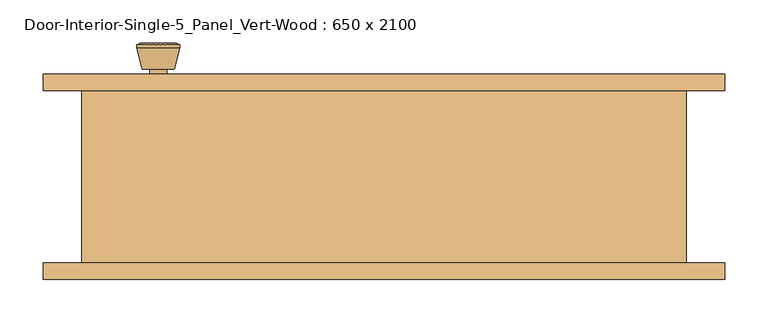
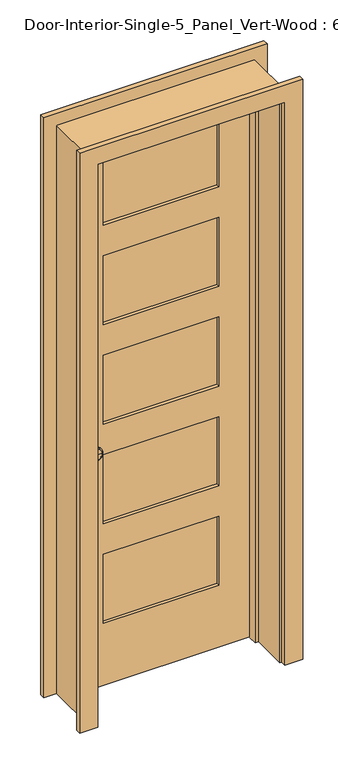
"""IFC4 building model written with IfcOpenShell, lengths in millimetres: door geometry, Door-Interior-Single-5_Panel_Vert-Wood : 650 x 2100."""

from ifc_helpers import new_model, si_unit, point, frame, frame_2d, origin, place, context, project, spatial, polyline, circle_curve, trimmed, segment, composite_curve, outline, extrude, faceted_brep, source, transform, mapped, element, save
from ifc_brep_helpers import plane_surface, cylinder_surface, revolved_surface, advanced_brep


def door_interior_single_5_panel_vert_wood_650_x_2100_a7f2c8da(model_context):
    return source(origin(), model_context, "Body", "SolidModel", [
        advanced_brep(
        [(-261.5, 55.9, 914.4), (-251.5, 55.9, 914.4), (-271.5, 55.9, 914.4), (-241.0241324, 6.9, 914.4), (-261.5, 6.9, 914.4), (-281.9758676, 6.9, 914.4), (-236.5, 8.7278681, 914.4), (-286.5, 8.7278681, 914.4), (-236.5, 12.1915463, 914.4), (-286.5, 12.1915463, 914.4), (-242.863764, 36.9, 914.4), (-280.136236, 36.9, 914.4), (-251.5, 36.9, 914.4), (-271.5, 36.9, 914.4)],
        [
            (0, 1),
            (1, 2, circle_curve(frame((-261.5, 55.9, 914.4), z_axis=(0.0, 1.0, 0.0), x_axis=(-1.0, 0.0, 0.0)), 10.0)),
            (2, 0),
            (2, 1, circle_curve(frame((-261.5, 55.9, 914.4), z_axis=(0.0, 1.0, 0.0), x_axis=(-1.0, 0.0, 0.0)), 10.0)),
            (3, 4),
            (4, 5),
            (5, 3, circle_curve(frame((-261.5, 6.9, 914.4), z_axis=(0.0, -1.0, 0.0), x_axis=(-1.0, 0.0, 0.0)), 20.4758676)),
            (3, 5, circle_curve(frame((-261.5, 6.9, 914.4), z_axis=(0.0, -1.0, 0.0), x_axis=(-1.0, 0.0, 0.0)), 20.4758676)),
            (6, 3),
            (5, 7),
            (7, 6, circle_curve(frame((-261.5, 8.7278681, 914.4), z_axis=(0.0, -1.0, 0.0), x_axis=(-1.0, 0.0, 0.0)), 25.0)),
            (6, 7, circle_curve(frame((-261.5, 8.7278681, 914.4), z_axis=(0.0, -1.0, 0.0), x_axis=(-1.0, 0.0, 0.0)), 25.0)),
            (8, 6),
            (7, 9),
            (9, 8, circle_curve(frame((-261.5, 12.1915463, 914.4), z_axis=(0.0, -1.0, 0.0), x_axis=(-1.0, 0.0, 0.0)), 25.0)),
            (8, 9, circle_curve(frame((-261.5, 12.1915463, 914.4), z_axis=(0.0, -1.0, 0.0), x_axis=(-1.0, 0.0, 0.0)), 25.0)),
            (10, 8),
            (9, 11),
            (11, 10, circle_curve(frame((-261.5, 36.9, 914.4), z_axis=(0.0, -1.0, 0.0), x_axis=(-1.0, 0.0, 0.0)), 18.636236)),
            (10, 11, circle_curve(frame((-261.5, 36.9, 914.4), z_axis=(0.0, -1.0, 0.0), x_axis=(-1.0, 0.0, 0.0)), 18.636236)),
            (12, 10),
            (11, 13),
            (13, 12, circle_curve(frame((-261.5, 36.9, 914.4), z_axis=(0.0, -1.0, 0.0), x_axis=(-1.0, 0.0, 0.0)), 10.0)),
            (12, 13, circle_curve(frame((-261.5, 36.9, 914.4), z_axis=(0.0, -1.0, 0.0), x_axis=(-1.0, 0.0, 0.0)), 10.0)),
            (1, 12),
            (13, 2),
        ],
        [
            plane_surface(frame((-261.5, 55.9, 914.4), z_axis=(0.0, 1.0, 0.0), x_axis=(-1.0, 0.0, 0.0))),
            plane_surface(frame((-261.5, 6.9, 914.4), z_axis=(0.0, -1.0, 0.0), x_axis=(-1.0, 0.0, 0.0))),
            revolved_surface(polyline([(-281.9758676, 6.9, 914.4), (-286.5, 8.7278681, 914.4)]), (-261.5, 55.9, 914.4), (0.0, 1.0, 0.0)),
            cylinder_surface(frame((-261.5, 55.9, 914.4), z_axis=(0.0, 1.0, 0.0), x_axis=(-1.0, 0.0, 0.0)), 25.0),
            revolved_surface(polyline([(-286.5, 12.1915463, 914.4), (-280.136236, 36.9, 914.4)]), (-261.5, 55.9, 914.4), (0.0, 1.0, 0.0)),
            plane_surface(frame((-261.5, 36.9, 914.4), z_axis=(0.0, 1.0, 0.0), x_axis=(-1.0, 0.0, 0.0))),
            cylinder_surface(frame((-261.5, 55.9, 914.4), z_axis=(0.0, 1.0, 0.0), x_axis=(-1.0, 0.0, 0.0)), 10.0),
        ],
        [
            (0, [[1, 2, 3]]),
            (0, [[-3, 4, -1]]),
            (1, [[5, 6, 7]]),
            (1, [[-6, -5, 8]]),
            (2, [[9, -7, 10, 11]]),
            (2, [[-10, -8, -9, 12]]),
            (3, [[13, -11, 14, 15]]),
            (3, [[-14, -12, -13, 16]]),
            (4, [[17, -15, 18, 19]]),
            (4, [[-18, -16, -17, 20]]),
            (5, [[21, -19, 22, 23]]),
            (5, [[-22, -20, -21, 24]]),
            (6, [[25, -23, 26, -2]]),
            (6, [[-26, -24, -25, -4]]),
        ],
    ),
        extrude(outline(composite_curve([segment(trimmed(circle_curve(frame_2d((914.4, -261.5)), 30.0), [point((914.4, -291.5))], [point((914.4, -231.5))], False, "CARTESIAN"), True, "CONTINUOUS"), segment(trimmed(circle_curve(frame_2d((914.4, -261.5)), 30.0), [point((914.4, -231.5))], [point((914.4, -291.5))], False, "CARTESIAN"), True, "CONTINUOUS")], self_intersect=False)), frame((0.0, 55.9, 0.0), z_axis=(0.0, 1.0, 0.0), x_axis=(0.0, 0.0, 1.0)), (0.0, 0.0, 1.0), 6.0),
        advanced_brep(
        [(-261.5, 102.825, 914.4), (-271.5, 102.825, 914.4), (-251.5, 102.825, 914.4), (-241.0241324, 151.825, 914.4), (-281.9758676, 151.825, 914.4), (-261.5, 151.825, 914.4), (-236.5, 149.9971319, 914.4), (-286.5, 149.9971319, 914.4), (-236.5, 146.5334537, 914.4), (-286.5, 146.5334537, 914.4), (-242.863764, 121.825, 914.4), (-280.136236, 121.825, 914.4), (-251.5, 121.825, 914.4), (-271.5, 121.825, 914.4)],
        [
            (0, 1),
            (1, 2, circle_curve(frame((-261.5, 102.825, 914.4), z_axis=(0.0, -1.0, 0.0), x_axis=(-1.0, 0.0, 0.0)), 10.0)),
            (2, 0),
            (2, 1, circle_curve(frame((-261.5, 102.825, 914.4), z_axis=(0.0, -1.0, 0.0), x_axis=(-1.0, 0.0, 0.0)), 10.0)),
            (3, 4, circle_curve(frame((-261.5, 151.825, 914.4), z_axis=(0.0, 1.0, 0.0), x_axis=(-1.0, 0.0, 0.0)), 20.4758676)),
            (4, 5),
            (5, 3),
            (4, 3, circle_curve(frame((-261.5, 151.825, 914.4), z_axis=(0.0, 1.0, 0.0), x_axis=(-1.0, 0.0, 0.0)), 20.4758676)),
            (6, 7, circle_curve(frame((-261.5, 149.9971319, 914.4), z_axis=(0.0, 1.0, 0.0), x_axis=(-1.0, 0.0, 0.0)), 25.0)),
            (7, 4),
            (3, 6),
            (7, 6, circle_curve(frame((-261.5, 149.9971319, 914.4), z_axis=(0.0, 1.0, 0.0), x_axis=(-1.0, 0.0, 0.0)), 25.0)),
            (8, 9, circle_curve(frame((-261.5, 146.5334537, 914.4), z_axis=(0.0, 1.0, 0.0), x_axis=(-1.0, 0.0, 0.0)), 25.0)),
            (9, 7),
            (6, 8),
            (9, 8, circle_curve(frame((-261.5, 146.5334537, 914.4), z_axis=(0.0, 1.0, 0.0), x_axis=(-1.0, 0.0, 0.0)), 25.0)),
            (10, 11, circle_curve(frame((-261.5, 121.825, 914.4), z_axis=(0.0, 1.0, 0.0), x_axis=(-1.0, 0.0, 0.0)), 18.636236)),
            (11, 9),
            (8, 10),
            (11, 10, circle_curve(frame((-261.5, 121.825, 914.4), z_axis=(0.0, 1.0, 0.0), x_axis=(-1.0, 0.0, 0.0)), 18.636236)),
            (12, 13, circle_curve(frame((-261.5, 121.825, 914.4), z_axis=(0.0, 1.0, 0.0), x_axis=(-1.0, 0.0, 0.0)), 10.0)),
            (13, 11),
            (10, 12),
            (13, 12, circle_curve(frame((-261.5, 121.825, 914.4), z_axis=(0.0, 1.0, 0.0), x_axis=(-1.0, 0.0, 0.0)), 10.0)),
            (1, 13),
            (12, 2),
        ],
        [
            plane_surface(frame((-261.5, 102.825, 914.4), z_axis=(0.0, -1.0, 0.0), x_axis=(-1.0, 0.0, 0.0))),
            plane_surface(frame((-261.5, 151.825, 914.4), z_axis=(0.0, 1.0, 0.0), x_axis=(-1.0, 0.0, 0.0))),
            revolved_surface(polyline([(-281.9758676, 151.825, 914.4), (-286.5, 149.9971319, 914.4)]), (-261.5, 102.825, 914.4), (0.0, -1.0, 0.0)),
            cylinder_surface(frame((-261.5, 102.825, 914.4), z_axis=(0.0, -1.0, 0.0), x_axis=(-1.0, 0.0, 0.0)), 25.0),
            revolved_surface(polyline([(-286.5, 146.5334537, 914.4), (-280.136236, 121.825, 914.4)]), (-261.5, 102.825, 914.4), (0.0, -1.0, 0.0)),
            plane_surface(frame((-261.5, 121.825, 914.4), z_axis=(0.0, -1.0, 0.0), x_axis=(-1.0, 0.0, 0.0))),
            cylinder_surface(frame((-261.5, 102.825, 914.4), z_axis=(0.0, -1.0, 0.0), x_axis=(-1.0, 0.0, 0.0)), 10.0),
        ],
        [
            (0, [[1, 2, 3]]),
            (0, [[-3, 4, -1]]),
            (1, [[5, 6, 7]]),
            (1, [[8, -7, -6]]),
            (2, [[9, 10, -5, 11]]),
            (2, [[12, -11, -8, -10]]),
            (3, [[13, 14, -9, 15]]),
            (3, [[16, -15, -12, -14]]),
            (4, [[17, 18, -13, 19]]),
            (4, [[20, -19, -16, -18]]),
            (5, [[21, 22, -17, 23]]),
            (5, [[24, -23, -20, -22]]),
            (6, [[-2, 25, -21, 26]]),
            (6, [[-4, -26, -24, -25]]),
        ],
    ),
        extrude(outline(composite_curve([segment(trimmed(circle_curve(frame_2d((914.4, -261.5)), 30.0), [point((914.4, -291.5))], [point((914.4, -231.5))], False, "CARTESIAN"), True, "CONTINUOUS"), segment(trimmed(circle_curve(frame_2d((914.4, -261.5)), 30.0), [point((914.4, -231.5))], [point((914.4, -291.5))], False, "CARTESIAN"), True, "CONTINUOUS")], self_intersect=False)), frame((0.0, 96.825, 0.0), z_axis=(0.0, 1.0, 0.0), x_axis=(0.0, 0.0, 1.0)), (0.0, 0.0, 1.0), 6.0),
        faceted_brep([(350.4, 96.825, 0.0), (350.4, -103.175, 0.0), (325.0, -103.175, 0.0), (325.0, 26.975, 0.0), (312.3, 26.975, 0.0), (312.3, 61.9, 0.0), (325.0, 61.9, 0.0), (325.0, 96.825, 0.0), (350.4, 96.825, 2125.4), (350.4, -103.175, 2125.4), (-350.4, -103.175, 2125.4), (-350.4, -103.175, 0.0), (-325.0, -103.175, 0.0), (-325.0, -103.175, 2100.0), (325.0, -103.175, 2100.0), (325.0, 26.975, 2100.0), (-325.0, 26.975, 2100.0), (-325.0, 26.975, 0.0), (-312.3, 26.975, 0.0), (-312.3, 26.975, 2087.3), (312.3, 26.975, 2087.3), (312.3, 61.9, 2087.3), (-312.3, 61.9, 2087.3), (-312.3, 61.9, 0.0), (-325.0, 61.9, 0.0), (-325.0, 61.9, 2100.0), (325.0, 61.9, 2100.0), (325.0, 96.825, 2100.0), (-325.0, 96.825, 2100.0), (-325.0, 96.825, 0.0), (-350.4, 96.825, 0.0), (-350.4, 96.825, 2125.4)], [[[0, 1, 2, 3, 4, 5, 6, 7]], [[1, 0, 8, 9]], [[2, 1, 9, 10, 11, 12, 13, 14]], [[3, 2, 14, 15]], [[4, 3, 15, 16, 17, 18, 19, 20]], [[5, 4, 20, 21]], [[6, 5, 21, 22, 23, 24, 25, 26]], [[7, 6, 26, 27]], [[0, 7, 27, 28, 29, 30, 31, 8]], [[9, 8, 31, 10]], [[15, 14, 13, 16]], [[21, 20, 19, 22]], [[27, 26, 25, 28]], [[30, 29, 24, 23, 18, 17, 12, 11]], [[10, 31, 30, 11]], [[16, 13, 12, 17]], [[22, 19, 18, 23]], [[28, 25, 24, 29]]]),
        extrude(outline(polyline([(2100.0, -325.0), (0.0, -325.0), (0.0, 325.0), (2100.0, 325.0), (2100.0, -325.0)]), holes=[polyline([(1980.9375, -204.35), (1980.9375, 204.35), (1722.545, 204.35), (1722.545, -204.35), (1980.9375, -204.35)]), polyline([(490.1675, -204.35), (490.1675, 204.35), (231.775, 204.35), (231.775, -204.35), (490.1675, -204.35)]), polyline([(1235.5525, -204.35), (1235.5525, 204.35), (977.16, 204.35), (977.16, -204.35), (1235.5525, -204.35)]), polyline([(1608.245, -204.35), (1608.245, 204.35), (1349.8525, 204.35), (1349.8525, -204.35), (1608.245, -204.35)]), polyline([(862.86, -204.35), (862.86, 204.35), (604.4675, 204.35), (604.4675, -204.35), (862.86, -204.35)])]), frame((0.0, 61.9, 0.0), z_axis=(0.0, 1.0, 0.0), x_axis=(0.0, 0.0, 1.0)), (0.0, 0.0, 1.0), 34.925),
        extrude(outline(polyline([(204.35, 73.5416667), (-204.35, 73.5416667), (-204.35, 85.1833333), (204.35, 85.1833333), (204.35, 73.5416667)])), frame((0.0, 0.0, 1722.545), z_axis=(0.0, 0.0, 1.0), x_axis=(1.0, 0.0, 0.0)), (0.0, 0.0, 1.0), 258.3925),
        extrude(outline(polyline([(204.35, 73.5416667), (-204.35, 73.5416667), (-204.35, 85.1833333), (204.35, 85.1833333), (204.35, 73.5416667)])), frame((0.0, 0.0, 1349.8525), z_axis=(0.0, 0.0, 1.0), x_axis=(1.0, 0.0, 0.0)), (0.0, 0.0, 1.0), 258.3925),
        extrude(outline(polyline([(204.35, 73.5416667), (-204.35, 73.5416667), (-204.35, 85.1833333), (204.35, 85.1833333), (204.35, 73.5416667)])), frame((0.0, 0.0, 604.4675), z_axis=(0.0, 0.0, 1.0), x_axis=(1.0, 0.0, 0.0)), (0.0, 0.0, 1.0), 258.3925),
        extrude(outline(polyline([(204.35, 73.5416667), (-204.35, 73.5416667), (-204.35, 85.1833333), (204.35, 85.1833333), (204.35, 73.5416667)])), frame((0.0, 0.0, 231.775), z_axis=(0.0, 0.0, 1.0), x_axis=(1.0, 0.0, 0.0)), (0.0, 0.0, 1.0), 258.3925),
        extrude(outline(polyline([(204.35, 73.5416667), (-204.35, 73.5416667), (-204.35, 85.1833333), (204.35, 85.1833333), (204.35, 73.5416667)])), frame((0.0, 0.0, 977.16), z_axis=(0.0, 0.0, 1.0), x_axis=(1.0, 0.0, 0.0)), (0.0, 0.0, 1.0), 258.3925),
        extrude(outline(polyline([(0.0, 331.35), (0.0, 394.85), (2169.85, 394.85), (2169.85, -394.85), (0.0, -394.85), (0.0, -331.35), (2106.35, -331.35), (2106.35, 331.35), (0.0, 331.35)])), frame((0.0, 96.825, 0.0), z_axis=(0.0, 1.0, 0.0), x_axis=(0.0, 0.0, 1.0)), (0.0, 0.0, 1.0), 19.05),
        extrude(outline(polyline([(0.0, 331.35), (0.0, 394.85), (2169.85, 394.85), (2169.85, -394.85), (0.0, -394.85), (0.0, -331.35), (2106.35, -331.35), (2106.35, 331.35), (0.0, 331.35)])), frame((0.0, -122.225, 0.0), z_axis=(0.0, 1.0, 0.0), x_axis=(0.0, 0.0, 1.0)), (0.0, 0.0, 1.0), 19.05),
    ])


if __name__ == "__main__":
    model = new_model("IFC4")
    model_context = context("Model", 3, world=origin())
    ifc_project = project(units=[si_unit("LENGTHUNIT", "METRE", prefix="MILLI")], contexts=[model_context])
    site = spatial("IfcSite", under=ifc_project)
    building = spatial("IfcBuilding", under=site)
    placement = place(None, origin())
    door_interior_single_5_panel_vert_wood_650_x_2100_shape = door_interior_single_5_panel_vert_wood_650_x_2100_a7f2c8da(model_context)
    element("IfcDoor", 1, ObjectType="Door-Interior-Single-5_Panel_Vert-Wood : 650 x 2100", at=placement, inside=building, context=model_context, shape_type="MappedRepresentation", body=[
        mapped(door_interior_single_5_panel_vert_wood_650_x_2100_shape, transform((0.0, 0.0, 0.0), x_axis=(1.0, 0.0, 0.0), y_axis=(0.0, 1.0, 0.0), z_axis=(0.0, 0.0, 1.0))),
    ])
    save(model, "model.ifc")

# Revit data of these elements
# Type "Door-Interior-Single-5_Panel_Vert-Wood : 650 x 2100"
#   Type Mark = "22"
#   Assembly Code = "C1020300"
#   Analytic Construction = "Wooden"
#   Top Rail = 0' - 4 11/16"
#   Thickness = 0' - 1 3/8"
#   Thermal Resistance (R) = 2.5876 (h·ft²·°F)/BTU
#   Swing Angle [instance default] = 90.00°
#   Stiles = 0' - 4 3/4"
#   Rough Width = 2' - 3.59055"
#   Rough Height = 6' - 11.67717"
#   Intermediate Rail = 0' - 4 1/2"
#   Height = 6' - 10.67717"
#   Width = 2' - 1.59055"
#   Heat Transfer Coefficient (U) = 0.3865 BTU/(h·ft²·°F)
#   Bottom Rail = 0' - 9 1/8"
#   Trim Material = Cherry
#   Panel Material = Cherry
#   Frame Material = Cherry
#   Door Handle Material = Aluminum
#   Visual Light Transmittance = 0
#   Solar Heat Gain Coefficient = 0
#   Wall Closure = (empty or 0)
#   Function = (empty or 0)
# Element 1 (IfcDoor, "Door-Interior-Single-5_Panel_Vert-Wood : 650 x 2100")
#   Materials on its faces: "Cherry", "Aluminum"
# Materials
#   "Cherry": class "Wood", colour RGB 226 177 128, transparency 0, Description = "Prunus Serotina", Cost = 0
#   "Aluminum": class "Metal", colour RGB 247 247 247, transparency 0, Description = "Aluminum 6061", Cost = 0
